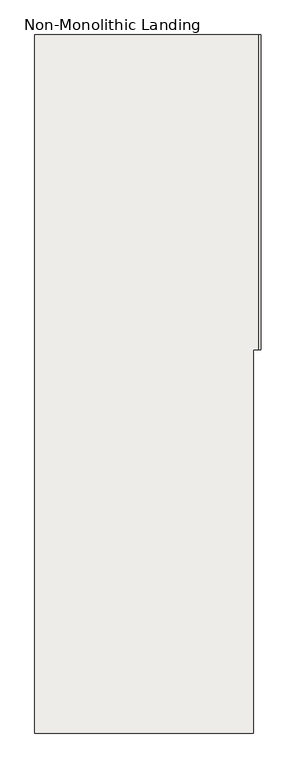
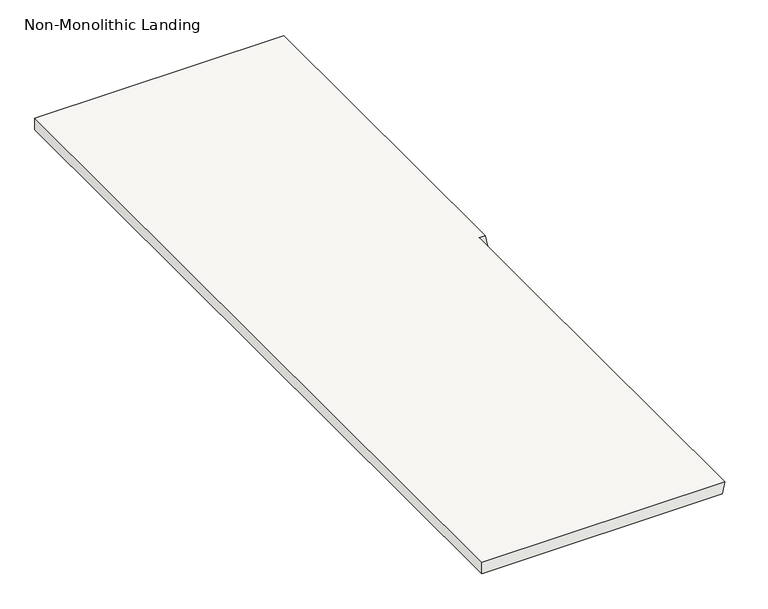
"""IFC4 building model written with IfcOpenShell, lengths in millimetres: slab geometry, Non-Monolithic Landing."""

from ifc_helpers import new_model, si_unit, origin, place, context, project, spatial, faceted_brep, source, transform, mapped, element, save


def non_monolithic_landing_e830aeb0(model_context):
    return source(origin(), model_context, "Body", "Brep", [
        faceted_brep([(-209.3966936, 601.2300402, 2000.0), (-200.0216936, 601.2300402, 1950.0), (-200.0216936, 2038.4290713, 1950.0), (-209.3966936, 2038.4290713, 2000.0), (-234.3966936, 215.3469597, 2000.0), (-234.3966936, 601.2300402, 2000.0), (-234.3966936, 2038.4290713, 2000.0), (-1234.4224748, 2038.4290713, 2000.0), (-1234.4224748, -1149.071626, 2000.0), (-234.3966936, -1149.071626, 2000.0), (-234.3966936, 601.2300402, 1950.0), (-234.3966936, 215.3469597, 1950.0), (-243.7716936, 215.3469597, 1950.0), (-243.7716936, -1149.071626, 1950.0), (-1234.4224748, -1149.071626, 1950.0), (-1234.4224748, 2038.4290713, 1950.0), (-234.3966936, 2038.4290713, 1950.0)], [[[0, 1, 2, 3]], [[4, 5, 0, 3, 6, 7, 8, 9]], [[10, 11, 12, 13, 14, 15, 16, 2, 1]], [[5, 4, 11, 10]], [[0, 5, 10, 1]], [[6, 3, 2, 16]], [[7, 6, 16, 15]], [[8, 7, 15, 14]], [[9, 8, 14, 13]], [[4, 12, 11]], [[12, 4, 9, 13]]]),
    ])


if __name__ == "__main__":
    model = new_model("IFC4")
    model_context = context("Model", 3, world=origin())
    ifc_project = project(units=[si_unit("LENGTHUNIT", "METRE", prefix="MILLI")], contexts=[model_context])
    site = spatial("IfcSite", under=ifc_project)
    building = spatial("IfcBuilding", under=site)
    placement = place(None, origin())
    non_monolithic_landing_shape = non_monolithic_landing_e830aeb0(model_context)
    element("IfcSlab", 1, ObjectType="Non-Monolithic Landing", at=placement, inside=building, context=model_context, shape_type="MappedRepresentation", body=[
        mapped(non_monolithic_landing_shape, transform((0.0, 0.0, 0.0), x_axis=(1.0, 0.0, 0.0), y_axis=(0.0, 1.0, 0.0), z_axis=(0.0, 0.0, 1.0))),
    ])
    save(model, "model.ifc")
